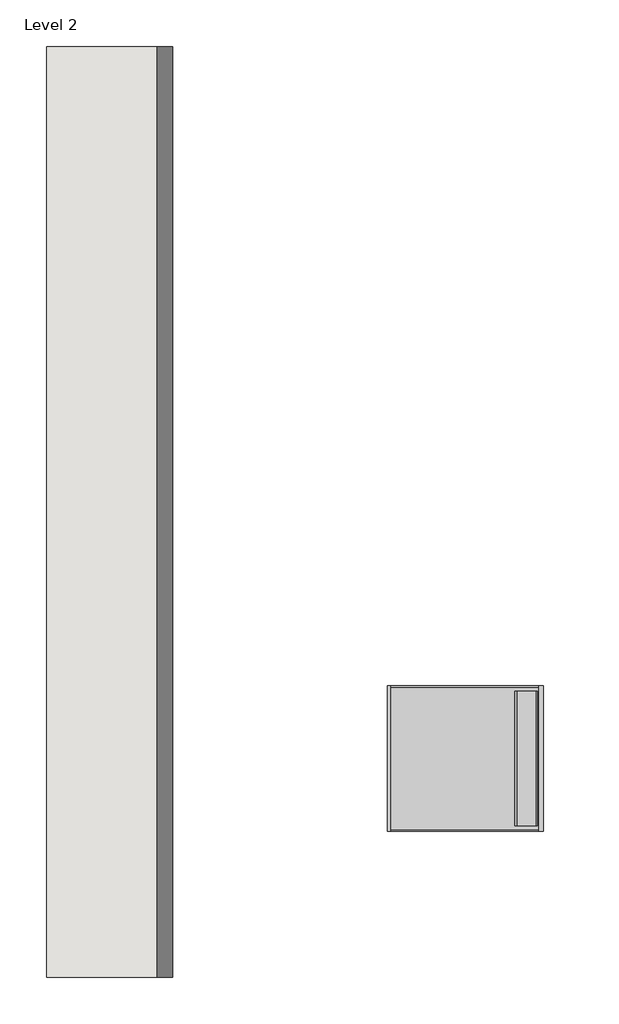
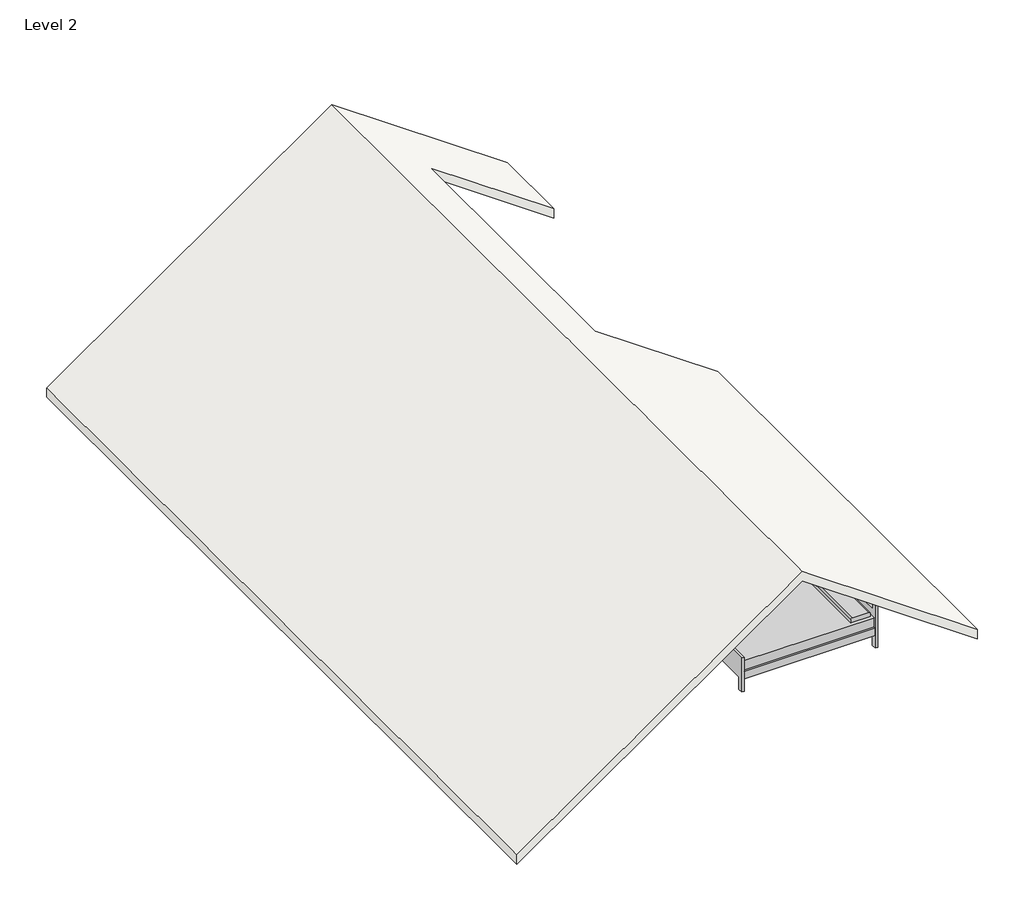
# One storey: 1 furniture element, 1 roof.
"""IFC4 building model written with IfcOpenShell, lengths in millimetres."""

from ifc_helpers import new_model, si_unit, origin, place, context, project, spatial, faceted_brep, transform, mapped, element, save
from components import furniture_b8e5f23d

model = new_model("IFC4")

# Units and contexts
model_context = context("Model", 3, world=origin())
ifc_project = project(units=[si_unit("LENGTHUNIT", "METRE", prefix="MILLI")], contexts=[model_context])

# Site, building, storey
site = spatial("IfcSite", under=ifc_project)
building = spatial("IfcBuilding", under=site)
storey = spatial("IfcBuildingStorey", under=building, Name="Level 2", Elevation=5000.0)

# Furniture
placement = place(None, origin())
furniture_shape = furniture_b8e5f23d(model_context)
element("IfcFurniture", 1, ObjectType="Bed-Shaker : King 78\" x 83\"", at=placement, inside=storey, context=model_context, shape_type="MappedRepresentation", body=[
    mapped(furniture_shape, transform((-1477.0000057, 10434.0490528, 5000.0), x_axis=(0.0, -1.0, 0.0), y_axis=(1.0, 0.0, 0.0), z_axis=(0.0, 0.0, 1.0))),
])

# Roof
element("IfcRoof", 2, ObjectType="Roof_Generic-125mm", at=placement, inside=storey, context=model_context, shape_type="Brep", body=[
    faceted_brep([(-8225.2000057, 7477.4990528, 5000.0), (-8225.2000057, 20132.4990528, 5000.0), (-3790.8112016, 20132.4990528, 8104.9924679), (-3790.8112016, 7477.4990528, 8104.9924679), (-1070.2000057, 20132.4990528, 6200.0), (-1070.2000057, 18874.9990528, 6200.0), (-2985.2000057, 18874.9990528, 7540.8974357), (-2985.2000057, 14459.9990528, 7540.8974357), (-1070.2000057, 14459.9990528, 6200.0), (-1070.2000057, 7477.4990528, 6200.0), (-8225.2000057, 20132.4990528, 5152.5968236), (-8225.2000057, 7477.4990528, 5152.5968236), (-3790.8112016, 7477.4990528, 8257.5892915), (-3790.8112016, 20132.4990528, 8257.5892915), (-1070.2000057, 20132.4990528, 6352.5968236), (-1070.2000057, 7477.4990528, 6352.5968236), (-1070.2000057, 14459.9990528, 6352.5968236), (-2985.2000057, 14459.9990528, 7693.4942593), (-2985.2000057, 18874.9990528, 7693.4942593), (-1070.2000057, 18874.9990528, 6352.5968236)], [[[0, 1, 2, 3]], [[2, 4, 5, 6, 7, 8, 9, 3]], [[10, 11, 12, 13]], [[14, 13, 12, 15, 16, 17, 18, 19]], [[0, 11, 10, 1]], [[8, 16, 15, 9]], [[4, 14, 19, 5]], [[10, 13, 14, 4, 2, 1]], [[17, 16, 8, 7]], [[18, 17, 7, 6]], [[19, 18, 6, 5]], [[15, 12, 11, 0, 3, 9]]]),
])

save(model, "model.ifc")

# Revit data of these elements
# Type "Bed-Shaker : King 78\" x 83\""
#   Assembly Code = "E2020200"
#   Length = 2108.2 mm
#   Width = 1981.2 mm
#   Frame Material = Birch
#   Mattress Material = Linen, White
#   Default Elevation = 0
# Type "Roof_Generic-125mm"
#   Layers, outside or top first: 125 mm no material (function 1)
# Element 1 (IfcFurniture, "Bed-Shaker : King 78\" x 83\"")
#   Phase Created = New Construction
#   Materials on its faces: "Birch", "Linen, White"
# Element 2 (IfcRoof, "Roof_Generic-125mm")
#   built-in parameter 1001705 = 27.0918 (stored number, unit not read)
#   built-in parameter 1001710 = 33615
#   Phase Created = New Construction
#   Materials on its faces: "Air"
# Materials
#   "Birch": class "Wood", colour RGB 224 178 126, transparency 0, Description = "Betula Alleghaniensis", Cost = 0
#   "Linen, White": class "Textile", colour RGB 247 247 239, transparency 0, Description = "Linen, white", Cost = 0
#   "Air": class "Gas", colour RGB 255 255 255, transparency 0, Description = "Air", Cost = 0
